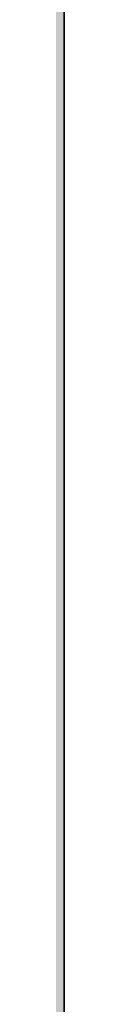
# Model space of a CAD drawing. Units: inches. Extents: x 2083 to 3317, y 1141 to 2115.
# Tile 236 of 256: x 3126.96 to 3126.96, y 1267.234 to 1271.372. Entities that reach past the tile are written whole.
import ezdxf

# ---------------------------------------------------------------- set-up
doc = ezdxf.new("R2010")
doc.units = ezdxf.units.IN
doc.layers.add('A-ANNO-DIMS', color=2, linetype='Continuous', lineweight=18)
doc.layers.add('A-WALL', color=7, linetype='Continuous', lineweight=35)
doc.layers.add('A-WALL-PATT', color=251, linetype='Continuous', lineweight=13, true_color=0x636466)
doc.styles.get("Standard").update_dxf_attribs({"font": 'arial.ttf'})
doc.dimstyles.new('ISO-25', dxfattribs={"dimtxt": 12, "dimasz": 12, "dimexe": 1.25, "dimexo": 0.625, "dimtad": 1, "dimlunit": 3, "dimtxsty": 'Standard', "dimcen": 2.5, "dimadec": 0, "dimazin": 0, "dimtfac": 1, "dimtmove": 0, "dimatfit": 3, "dimfxl": 1, "dimarcsym": 0})

# ---------------------------------------------------------------- blocks, each defined once
blk = doc.blocks.new('*D9')
at = {"layer": 'A-ANNO-DIMS', "color": 0, "lineweight": -2, "transparency": 16777216}
for p, q in [((3127.5848, 1486.7614), (3190.4031, 1486.7614)), ((3189.1531, 1474.7614), (3189.1531, 1275.2614)), ((3127.5848, 1263.2614), (3190.4031, 1263.2614))]:
    blk.add_line(p, q, dxfattribs=at)
at = {"layer": 'A-ANNO-DIMS', "color": 0, "transparency": 16777216}
for points in [[(3187.1531, 1474.7614), (3191.1531, 1474.7614), (3189.1531, 1486.7614)], [(3187.1531, 1275.2614), (3191.1531, 1275.2614), (3189.1531, 1263.2614)]]:
    blk.add_solid(points, dxfattribs=at)
at = {"layer": 'Defpoints', "color": 0, "transparency": 16777216}
for p in [(3126.9598, 1486.7614), (3126.9598, 1263.2614), (3189.1531, 1263.2614)]:
    blk.add_point(p, dxfattribs=at)
at = {"layer": 'A-ANNO-DIMS', "color": 0, "transparency": 16777216, "insert": (3182.4012, 1375.0114), "char_height": 12, "attachment_point": 5, "rotation": 90}
blk.add_mtext('18\'-7.5"', dxfattribs=at)
blk = doc.blocks.new('*D26')
at = {"layer": 'A-ANNO-DIMS', "color": 0, "lineweight": -2, "transparency": 16777216}
for p, q in [((3088.9858, 1274.9151), (3088.9858, 1270.952)), ((3111.24, 1274.9151), (3111.24, 1270.952)), ((3076.9858, 1272.202), (2840.2624, 1272.202)), ((3111.24, 1272.202), (3088.9858, 1272.202)), ((3123.24, 1272.202), (3135.24, 1272.202))]:
    blk.add_line(p, q, dxfattribs=at)
at = {"layer": 'A-ANNO-DIMS', "color": 0, "transparency": 16777216}
for points in [[(3076.9858, 1274.202), (3076.9858, 1270.202), (3088.9858, 1272.202)], [(3123.24, 1274.202), (3123.24, 1270.202), (3111.24, 1272.202)]]:
    blk.add_solid(points, dxfattribs=at)
at = {"layer": 'Defpoints', "color": 0, "transparency": 16777216}
for p in [(3088.9858, 1275.5401), (3111.24, 1275.5401), (3088.9858, 1272.202)]:
    blk.add_point(p, dxfattribs=at)
at = {"layer": 'A-ANNO-DIMS', "color": 0, "transparency": 16777216, "insert": (2952.6241, 1279.0316), "char_height": 12, "attachment_point": 5}
blk.add_mtext('NIGHTSTAND 1\'-10 1/2" TYP.', dxfattribs=at)
blk = doc.blocks.new('*D27')
at = {"layer": 'A-ANNO-DIMS', "color": 0, "lineweight": -2, "transparency": 16777216}
for p, q in [((3114.5782, 1309.7943), (3114.5782, 1321.7943)), ((3111.865, 1297.7943), (3115.8282, 1297.7943)), ((3114.5782, 1297.7943), (3114.5782, 1275.5401)), ((3111.865, 1275.5401), (3115.8282, 1275.5401)), ((3114.5782, 1263.5401), (3114.5782, 1140.9886))]:
    blk.add_line(p, q, dxfattribs=at)
at = {"layer": 'A-ANNO-DIMS', "color": 0, "transparency": 16777216}
for points in [[(3112.5782, 1309.7943), (3116.5782, 1309.7943), (3114.5782, 1297.7943)], [(3112.5782, 1263.5401), (3116.5782, 1263.5401), (3114.5782, 1275.5401)]]:
    blk.add_solid(points, dxfattribs=at)
at = {"layer": 'Defpoints', "color": 0, "transparency": 16777216}
for p in [(3111.24, 1297.7943), (3111.24, 1275.5401), (3114.5782, 1275.5401)]:
    blk.add_point(p, dxfattribs=at)
at = {"layer": 'A-ANNO-DIMS', "color": 0, "transparency": 16777216, "insert": (3107.7485, 1196.2643), "char_height": 12, "attachment_point": 5, "rotation": 90}
blk.add_mtext('1\'-10 1/2" TYP.', dxfattribs=at)

msp = doc.modelspace()

# ---------------------------------------------------------------- hatches: boundary and pattern name
at = {"layer": 'A-WALL-PATT'}
h = msp.add_hatch(color=256, dxfattribs=at)
h.dxf.hatch_style = 1
h.paths.add_polyline_path([(3126.9598, 2020.7614), (2748.9598, 2020.7614), (2604.9598, 2020.7614), (2226.9598, 2020.7614), (2226.9598, 1702.7614), (2466.9598, 1702.7614), (2466.9598, 1582.7614), (2418.9598, 1582.7614), (2418.9598, 1477.7614), (2226.9598, 1477.7614), (2226.9598, 1263.2614), (2544.9598, 1263.2614), (2544.9598, 1411.7614), (2604.9598, 1411.7614), (2685.9598, 1411.7614), (2685.9598, 1420.7614), (2604.9598, 1420.7614), (2604.9598, 1573.7614), (2604.9598, 1702.7614), (2604.9598, 2011.7614), (2748.9598, 2011.7614), (2748.9598, 1702.7614), (2862.9598, 1702.7614), (2862.9598, 1621.7614), (2871.9598, 1621.7614), (2871.9598, 1702.7614), (2883.9598, 1702.7614), (2883.9598, 1706.9395, -0.026459), (2883.9598, 1711.7614), (2757.9598, 1711.7614), (2757.9598, 1807.7614), (2787.9598, 1807.7614), (2787.9598, 1812.2614), (2757.9598, 1812.2614), (2757.9598, 2011.7614), (2877.9598, 2011.7614), (2877.9598, 1812.2614), (2847.9598, 1812.2614), (2847.9598, 1807.7614), (2889.8357, 1807.7614), (2889.8357, 1812.2614), (2882.4598, 1812.2614), (2882.4598, 2011.7614), (3117.9598, 2011.7614), (3117.9598, 1812.2614), (2937.8357, 1812.2614), (2937.8357, 1807.7614), (2995.7098, 1807.7614), (2995.7098, 1796.1177), (3000.2098, 1796.1177), (3000.2098, 1807.7614), (3117.9598, 1807.7614), (3117.9598, 1711.7614), (3000.2098, 1711.7614), (3000.2098, 1760.1177), (2998.5727, 1760.1177, -0.020711), (2995.7098, 1760.1177), (2995.7098, 1711.7614), (2931.9598, 1711.7614), (2931.9598, 1702.7614), (3126.9598, 1702.7614)])
h.paths.add_polyline_path([(2471.4598, 2011.7614), (2471.4598, 1810.0114), (2462.7169, 1810.0114), (2462.7169, 1805.5114), (2505.9598, 1805.5114), (2505.9598, 1810.0114), (2475.9598, 1810.0114), (2475.9598, 2011.7614), (2595.9598, 2011.7614), (2595.9598, 1810.0114), (2565.9598, 1810.0114), (2565.9598, 1805.5114), (2595.9598, 1805.5114), (2595.9598, 1711.7614), (2235.9598, 1711.7614), (2235.9598, 1805.5114), (2353.7098, 1805.5114), (2353.7098, 1796.0542), (2358.2098, 1796.0542), (2358.2098, 1805.5114), (2414.7169, 1805.5114), (2414.7169, 1810.0114), (2235.9598, 1810.0114), (2235.9598, 2011.7614)], flags=16)
h.paths.add_polyline_path([(2270.2047, 1994.61), (2270.2047, 1970.61), (2246.2047, 1970.61), (2246.2047, 1994.61)], flags=0)
edge = h.paths.add_edge_path(flags=0)
edge.add_ellipse((2332.0274, 1899.7982), major_axis=(-3.043, 3.043), ratio=0.168252, start_angle=-161.3322, end_angle=-156.3071, ccw=False)
edge.add_ellipse((2333.082, 1898.7435), major_axis=(-1.0546, 1.0546), ratio=0.453532, start_angle=-123.371, end_angle=-94.1591)
edge = h.paths.add_edge_path(flags=0)
edge.add_ellipse((2332.0274, 1968.8763), major_axis=(3.043, 3.043), ratio=0.168252, start_angle=18.6678, end_angle=23.6929)
edge.add_spline(control_points=[(2332.9256, 1970.6911), (2332.2268, 1970.3361), (2330.8937, 1969.6589), (2328.4131, 1970.9321), (2327.2039, 1967.7487), (2324.7096, 1969.9556), (2322.5328, 1967.0124), (2320.0128, 1971.2958), (2317.6803, 1968.1578), (2316.0405, 1967.102), (2315.4269, 1966.8096)], knot_values=[0, 0, 0, 0, 2.267059, 4.324559, 6.685584, 8.878641, 11.121502, 14.300359, 17.755284, 19.732645, 19.732645, 19.732645, 19.732645], degree=3, periodic=0)
edge.add_ellipse((2332.0274, 1968.8763), major_axis=(3.043, 3.043), ratio=0.168252, start_angle=18.6678, end_angle=23.6929, ccw=False)
edge.add_ellipse((2333.082, 1969.9309), major_axis=(1.0546, 1.0546), ratio=0.453532, start_angle=56.629, end_angle=85.8409, ccw=False)
edge = h.paths.add_edge_path(flags=0)
edge.add_spline(control_points=[(2296.4283, 1967.9879), (2293.6278, 1965.3363), (2287.7036, 1959.7271), (2299.7439, 1949.9957), (2294.5326, 1935.6685), (2290.5732, 1920.6035), (2293.3941, 1909.9737), (2296.1854, 1904.9665)], knot_values=[0.099185, 0.099185, 0.099185, 0.099185, 0.345301, 0.619822, 0.982653, 1.386093, 1.810555, 1.810555, 1.810555, 1.810555], degree=3, periodic=0)
edge.add_spline(control_points=[(2296.1854, 1904.9665), (2297.3836, 1902.6193), (2298.001, 1901.9493), (2298.553, 1901.4682)], knot_values=[0.006246, 0.006246, 0.006246, 0.006246, 0.055476, 0.055476, 0.055476, 0.055476], degree=3, periodic=0)
edge.add_spline(control_points=[(2298.553, 1901.4682), (2297.2586, 1900.9232), (2295.2253, 1900.2321), (2293.0602, 1900.6142), (2292.1014, 1900.7884), (2292.0896, 1900.7906)], knot_values=[0.312835, 0.312835, 0.312835, 0.312835, 0.40178, 0.474987, 0.475903, 0.475903, 0.475903, 0.475903], degree=3, periodic=0)
edge.add_arc((2292.7936, 1904.6641), 3.937, 215.4209, 259.6982, ccw=False)
edge.add_spline(control_points=[(2289.5853, 1902.3823), (2289.4767, 1902.5351), (2289.3685, 1902.688), (2289.2609, 1902.8412)], knot_values=[0.102872, 0.102872, 0.102872, 0.102872, 0.116896, 0.116896, 0.116896, 0.116896], degree=3, periodic=0)
edge.add_spline(control_points=[(2289.2609, 1902.8412), (2288.6866, 1902.5502), (2287.64, 1902.0199), (2285.8813, 1901.874), (2283.853, 1901.5044), (2281.72, 1899.7105), (2278.467, 1899.4929), (2276.1571, 1901.8832), (2272.259, 1899.8041), (2267.7776, 1901.8432), (2262.2439, 1900.184), (2257.4149, 1901.7821), (2254.3184, 1900.7261), (2253.1783, 1900.3373)], knot_values=[0, 0, 0, 0, 1.907977, 3.477176, 5.261074, 7.972851, 11.680248, 13.717921, 16.939592, 22.789562, 27.502503, 33.595215, 37.145618, 37.145618, 37.145618, 37.145618], degree=3, periodic=0)
edge.add_line((2253.1783, 1900.3373), (2250.2442, 1902.8412))
edge.add_line((2250.2442, 1902.8412), (2250.2442, 1965.8333))
edge.add_line((2250.2442, 1965.8333), (2253.1783, 1968.3371))
edge.add_spline(control_points=[(2253.1783, 1968.3371), (2254.3184, 1967.9483), (2257.4149, 1966.8924), (2262.2439, 1968.4904), (2267.7776, 1966.8313), (2271.5267, 1968.5372), (2273.8759, 1967.8283), (2274.2067, 1967.7276)], knot_values=[0, 0, 0, 0, 0.09018, 0.244935, 0.364644, 0.513233, 0.537855, 0.537855, 0.537855, 0.537855], degree=3, periodic=0)
edge.add_arc((2274.3529, 1963.7933), 3.937, 72.0511, 92.1279, ccw=False)
edge.add_arc((2281.2969, 1985.23), 18.5963, 252.05113, 288.56572)
edge.add_arc((2292.3167, 1956.0289), 12.6461, 71.02679, 113.77822, ccw=False)
edge = h.paths.add_edge_path(flags=0)
edge.add_spline(control_points=[(2274.8994, 1951.8562), (2275.0662, 1951.6166), (2275.2327, 1951.3766), (2275.398, 1951.1359)], knot_values=[1.409916, 1.409916, 1.409916, 1.409916, 1.43159, 1.43159, 1.43159, 1.43159], degree=3, periodic=0)
edge.add_spline(control_points=[(2275.398, 1951.1359), (2275.7921, 1950.5619), (2276.1792, 1949.9838), (2276.5455, 1949.3971)], knot_values=[1.358238, 1.358238, 1.358238, 1.358238, 1.409916, 1.409916, 1.409916, 1.409916], degree=3, periodic=0)
edge.add_line((2276.5455, 1949.3971), (2277.4373, 1947.8622))
edge.add_spline(control_points=[(2277.4373, 1947.8622), (2276.3038, 1945.6731), (2274.6397, 1942.4269), (2274.6316, 1938.0939), (2272.7991, 1930.8515), (2274.3564, 1943.897), (2275.9477, 1947.9234), (2276.5455, 1949.3971)], knot_values=[0.005632, 0.005632, 0.005632, 0.005632, 0.186014, 0.266002, 0.357087, 0.59639, 0.739732, 0.739732, 0.739732, 0.739732], degree=3, periodic=0)
edge.add_spline(control_points=[(2276.5455, 1949.3971), (2276.1792, 1949.9838), (2275.7921, 1950.5619), (2275.398, 1951.1359)], knot_values=[1.358238, 1.358238, 1.358238, 1.358238, 1.409916, 1.409916, 1.409916, 1.409916], degree=3, periodic=0)
edge.add_spline(control_points=[(2275.398, 1951.1359), (2274.9425, 1950.0805), (2274.2078, 1948.0253), (2273.9346, 1944.8515), (2272.4685, 1937.6275), (2273.4662, 1945.6965), (2274.7006, 1951.0595), (2274.8994, 1951.8562)], knot_values=[0.104364, 0.104364, 0.104364, 0.104364, 0.189636, 0.269624, 0.36071, 0.600013, 0.644622, 0.644622, 0.644622, 0.644622], degree=3, periodic=0)
h.paths.add_polyline_path([(2269.1675, 1963.1276, -0.357527), (2268.1706, 1960.9764, -0.092561), (2268.1706, 1939.4363, -0.357527), (2269.1675, 1937.2851, -0.357527), (2267.0163, 1938.282, -0.164785), (2254.6856, 1938.282, -0.357527), (2252.5344, 1937.2851, -0.357527), (2253.5313, 1939.4363, -0.092561), (2253.5313, 1960.9764, -0.357527), (2252.5344, 1963.1276, -0.357527), (2254.6856, 1962.1307, -0.164785), (2267.0163, 1962.1307, -0.357527)], flags=0)
h.paths.add_polyline_path([(2248.8741, 1967.8018), (2248.8741, 1957.0277), (2249.4578, 1957.0277), (2249.4578, 1911.6468), (2248.8741, 1911.6468), (2248.8741, 1900.8727), (2246.5119, 1900.8727, 0.197327), (2244.1497, 1902.4569), (2244.1497, 1966.2176, 0.197327), (2246.5119, 1967.8018)], flags=0)
h.paths.add_polyline_path([(2269.1675, 1931.3893, -0.357527), (2268.1706, 1929.2381, -0.092561), (2268.1706, 1907.6981, -0.357527), (2269.1675, 1905.5469, -0.357527), (2267.0163, 1906.5438, -0.164785), (2254.6856, 1906.5438, -0.357527), (2252.5344, 1905.5469, -0.357527), (2253.5313, 1907.6981, -0.092561), (2253.5313, 1929.2381, -0.357527), (2252.5344, 1931.3893, -0.357527), (2254.6856, 1930.3925, -0.164785), (2267.0163, 1930.3925, -0.357527)], flags=0)
edge = h.paths.add_edge_path(flags=0)
edge.add_spline(control_points=[(2276.1969, 1906.7237), (2276.1681, 1909.0289), (2276.114, 1913.3719), (2270.5984, 1924.925), (2273.9052, 1919.0128), (2275.9217, 1916.2621), (2275.4746, 1912.4021), (2277.2579, 1910.3806), (2276.696, 1908.225), (2276.6462, 1906.813), (2276.6178, 1906.0084)], knot_values=[0, 0, 0, 0, 8.61026, 16.221274, 18.843057, 23.804898, 27.440828, 29.356102, 31.203478, 33.650687, 33.650687, 33.650687, 33.650687], degree=3, periodic=0)
edge.add_spline(control_points=[(2276.6178, 1906.0084), (2276.6233, 1905.6241), (2276.4977, 1904.6287), (2275.4418, 1903.8547), (2274.9373, 1903.0804), (2274.8591, 1902.8412)], knot_values=[0.156488, 0.156488, 0.156488, 0.156488, 0.184398, 0.231376, 0.250598, 0.250598, 0.250598, 0.250598], degree=3, periodic=0)
edge.add_line((2274.8591, 1902.8412), (2276.506, 1902.8412))
edge.add_spline(control_points=[(2276.506, 1902.8412), (2276.7883, 1903.0849), (2277.6651, 1904.1252), (2278.2495, 1904.3407), (2277.6539, 1908.5274), (2278.1557, 1906.2278), (2278.1005, 1905.2859), (2278.8467, 1904.069), (2277.8568, 1903.4149), (2277.8742, 1902.991), (2277.9036, 1902.8412)], knot_values=[0.059574, 0.059574, 0.059574, 0.059574, 0.080753, 0.103741, 0.16972, 0.176036, 0.207137, 0.240474, 0.262341, 0.27366, 0.27366, 0.27366, 0.27366], degree=3, periodic=0)
edge.add_line((2277.9036, 1902.8412), (2280.0298, 1902.8412))
edge.add_spline(control_points=[(2280.0298, 1902.8412), (2279.8882, 1903.0884), (2279.4993, 1903.9816), (2280.1523, 1905.9393), (2278.1036, 1909.6578), (2279.7624, 1907.1853), (2280.3279, 1904.8749), (2280.4851, 1903.4896), (2281.4633, 1903.2494), (2281.7583, 1902.9365), (2281.834, 1902.8412)], knot_values=[0.013856, 0.013856, 0.013856, 0.013856, 0.034874, 0.088867, 0.107879, 0.126738, 0.158714, 0.193757, 0.217487, 0.226722, 0.226722, 0.226722, 0.226722], degree=3, periodic=0)
edge.add_spline(control_points=[(2281.834, 1902.8412), (2281.7875, 1902.8267), (2281.647, 1902.783), (2281.3955, 1902.8595), (2281.0881, 1902.9852), (2280.7207, 1903.0609), (2280.3335, 1903.0257), (2280.1248, 1902.8989), (2280.0298, 1902.8412)], knot_values=[0, 0, 0, 0, 0.14413, 0.435517, 0.749276, 1.153046, 1.548371, 1.878348, 1.878348, 1.878348, 1.878348], degree=3, periodic=0)
edge.add_line((2280.0298, 1902.8412), (2277.9036, 1902.8412))
edge.add_spline(control_points=[(2277.9036, 1902.8412), (2277.8929, 1902.7959), (2277.8654, 1902.6796), (2277.6075, 1902.6875), (2277.2741, 1902.8007), (2276.8379, 1902.6198), (2276.5838, 1902.7893), (2276.506, 1902.8412)], knot_values=[0, 0, 0, 0, 0.127189, 0.326199, 0.628009, 1.24357, 1.515331, 1.515331, 1.515331, 1.515331], degree=3, periodic=0)
edge.add_line((2276.506, 1902.8412), (2274.8591, 1902.8412))
edge.add_spline(control_points=[(2274.8591, 1902.8412), (2274.8144, 1902.8986), (2274.7251, 1903.0134), (2274.4935, 1903.119), (2274.2443, 1902.9605), (2273.9371, 1903.1849), (2273.614, 1902.9831), (2273.4083, 1902.883), (2273.3223, 1902.8412)], knot_values=[0, 0, 0, 0, 0.21843, 0.436957, 0.687977, 0.990379, 1.398396, 1.69185, 1.69185, 1.69185, 1.69185], degree=3, periodic=0)
edge.add_spline(control_points=[(2273.3223, 1902.8412), (2273.6167, 1903.4457), (2274.274, 1904.5383), (2276.0272, 1904.5737), (2276.207, 1906.5836), (2276.1969, 1906.7237)], knot_values=[0.012227, 0.012227, 0.012227, 0.012227, 0.059472, 0.106218, 0.134458, 0.134458, 0.134458, 0.134458], degree=3, periodic=0)
h.paths.add_polyline_path([(2270.7761, 1897.7898), (2270.7761, 1873.7898), (2246.7761, 1873.7898), (2246.7761, 1897.7898)], flags=0)
h.paths.add_polyline_path([(2353.7098, 1760.0051), (2353.7098, 1760.0542), (2358.2098, 1760.0542, -0.033729)], flags=0)
h.paths.add_polyline_path([(2321.8191, 1737.5292), (2341.9953, 1737.5292, -0.414214), (2343.2033, 1736.3212), (2343.2033, 1721.0206, -0.414214), (2341.9953, 1719.8127), (2321.8191, 1719.8127, -0.414214), (2320.6112, 1721.0206), (2320.6112, 1736.3212, -0.414214)], flags=0)
h.paths.add_polyline_path([(2324.235, 1736.3212), (2339.5794, 1736.3212, -0.414214), (2341.9953, 1733.9053), (2341.9953, 1725.4497, -0.414214), (2339.5794, 1723.0338), (2333.6806, 1723.0338), (2333.8453, 1722.0455, -0.870646), (2335.4254, 1721.8259, -0.767327), (2333.9227, 1721.4232), (2331.291, 1721.4232, -0.767327), (2329.7883, 1721.8259, -0.870646), (2331.3684, 1722.0455), (2331.5331, 1723.0338), (2324.235, 1723.0338, -0.414214), (2321.8191, 1725.4497), (2321.8191, 1733.9053, -0.414214)], flags=0)
h.paths.add_polyline_path([(2570.4838, 1928.6154), (2589.6838, 1928.6154), (2590.1688, 1928.6154), (2590.1688, 1904.9934), (2570.4838, 1904.9934)], flags=0)
h.paths.add_polyline_path([(2574.4473, 1927.2638, -1), (2572.8288, 1927.2638, -1)], flags=0)
h.paths.add_polyline_path([(2573.0899, 1926.9409), (2573.925, 1927.776), (2574.1477, 1927.5533), (2573.3126, 1926.7182)], flags=0)
h.paths.add_polyline_path([(2578.7791, 1919.7296, -1), (2571.5917, 1919.7296, -1)], flags=0)
h.paths.add_polyline_path([(2578.3854, 1919.7296, -1), (2571.9854, 1919.7296, -1)], flags=0)
h.paths.add_polyline_path([(2331.5958, 1729.4762, -1), (2333.618, 1729.4762, -1)], flags=0)
h.paths.add_polyline_path([(2578.0342, 1927.2638, -1), (2576.4157, 1927.2638, -1)], flags=0)
h.paths.add_polyline_path([(2576.6889, 1927.5311), (2576.9116, 1927.7538), (2577.7467, 1926.9186), (2577.524, 1926.6959)], flags=0)
h.paths.add_polyline_path([(2578.1391, 1909.8595, -1), (2572.2317, 1909.8595, -1)], flags=0)
h.paths.add_polyline_path([(2577.7454, 1909.8595, -1), (2572.6254, 1909.8595, -1)], flags=0)
h.paths.add_polyline_path([(2583.7977, 1927.2638, -1), (2582.1792, 1927.2638, -1)], flags=0)
h.paths.add_polyline_path([(2582.7186, 1927.7538), (2583.5538, 1926.9186), (2583.3311, 1926.6959), (2582.4959, 1927.5311)], flags=0)
h.paths.add_polyline_path([(2582.4959, 1927.5311), (2582.7186, 1927.7538), (2583.5538, 1926.9186), (2583.3311, 1926.6959)], flags=0)
h.paths.add_polyline_path([(2587.7391, 1920.5296, -1), (2581.8317, 1920.5296, -1)], flags=0)
h.paths.add_polyline_path([(2587.3454, 1920.5296, -1), (2582.2254, 1920.5296, -1)], flags=0)
h.paths.add_polyline_path([(2587.3846, 1927.2638, -1), (2585.7661, 1927.2638, -1)], flags=0)
h.paths.add_polyline_path([(2586.082, 1926.9802), (2586.9172, 1927.8154), (2587.1399, 1927.5927), (2586.3047, 1926.7575)], flags=0)
h.paths.add_polyline_path([(2588.3791, 1910.6595, -1), (2581.1917, 1910.6595, -1)], flags=0)
h.paths.add_polyline_path([(2587.9854, 1910.6595, -1), (2581.5854, 1910.6595, -1)], flags=0)
h.paths.add_polyline_path([(2417.1677, 1729.4779), (2437.3439, 1729.4779, -0.414214), (2438.5519, 1728.2699), (2438.5519, 1712.9693, -0.414214), (2437.3439, 1711.7614), (2417.1677, 1711.7614, -0.414214), (2415.9598, 1712.9693), (2415.9598, 1728.2699, -0.414214)], flags=0)
h.paths.add_polyline_path([(2419.5836, 1728.2699), (2434.928, 1728.2699, -0.414214), (2437.3439, 1725.8541), (2437.3439, 1717.3984, -0.414214), (2434.928, 1714.9825), (2429.0292, 1714.9825), (2429.1939, 1713.9942, -0.870646), (2430.774, 1713.7746, -0.767327), (2429.2713, 1713.372), (2426.6396, 1713.372, -0.767327), (2425.1369, 1713.7746, -0.870646), (2426.717, 1713.9942), (2426.8817, 1714.9825), (2419.5836, 1714.9825, -0.414214), (2417.1677, 1717.3984), (2417.1677, 1725.8541, -0.414214)], flags=0)
h.paths.add_polyline_path([(2419.5836, 1728.2699), (2434.928, 1728.2699, -0.414214), (2437.3439, 1725.8541), (2437.3439, 1717.3984, -0.414214), (2434.928, 1714.9825), (2429.0292, 1714.9825), (2428.3581, 1719.009), (2427.5528, 1719.009), (2426.8817, 1714.9825), (2419.5836, 1714.9825, -0.414214), (2417.1677, 1717.3984), (2417.1677, 1725.8541, -0.414214)], flags=0)
h.paths.add_polyline_path([(2426.9444, 1721.4249, -1), (2428.9666, 1721.4249, -1)], flags=0)
h.paths.add_polyline_path([(2475.9598, 1702.7614), (2595.9598, 1702.7614), (2595.9598, 1582.7614), (2475.9598, 1582.7614)], flags=16)
h.paths.add_polyline_path([(2427.9598, 1573.7614), (2595.9598, 1573.7614), (2595.9598, 1468.7614), (2595.9598, 1420.7614), (2384.4598, 1420.7614), (2384.4598, 1468.7614), (2427.9598, 1468.7614)], flags=16)
h.paths.add_polyline_path([(2379.9598, 1468.7614), (2379.9598, 1420.7614), (2235.9598, 1420.7614), (2235.9598, 1468.7614)], flags=16)
h.paths.add_polyline_path([(2317.816, 1466.6958), (2337.9922, 1466.6958, -0.414214), (2339.2002, 1465.4878), (2339.2002, 1450.1872, -0.414214), (2337.9922, 1448.9792), (2317.816, 1448.9792, -0.414214), (2316.6081, 1450.1872), (2316.6081, 1465.4878, -0.414214)], flags=0)
h.paths.add_polyline_path([(2320.2319, 1465.4878), (2335.5763, 1465.4878, -0.414214), (2337.9922, 1463.0719), (2337.9922, 1454.6163, -0.414214), (2335.5763, 1452.2004), (2329.6775, 1452.2004), (2329.8422, 1451.212, -0.870646), (2331.4223, 1450.9925, -0.767327), (2329.9196, 1450.5898), (2327.2879, 1450.5898, -0.767327), (2325.7852, 1450.9925, -0.870646), (2327.3653, 1451.212), (2327.53, 1452.2004), (2320.2319, 1452.2004, -0.414214), (2317.816, 1454.6163), (2317.816, 1463.0719, -0.414214)], flags=0)
h.paths.add_polyline_path([(2320.2319, 1465.4878), (2335.5763, 1465.4878, -0.414214), (2337.9922, 1463.0719), (2337.9922, 1454.6163, -0.414214), (2335.5763, 1452.2004), (2329.6775, 1452.2004), (2329.0064, 1456.2269), (2328.2011, 1456.2269), (2327.53, 1452.2004), (2320.2319, 1452.2004, -0.414214), (2317.816, 1454.6163), (2317.816, 1463.0719, -0.414214)], flags=0)
h.paths.add_polyline_path([(2327.5926, 1458.6428, -1), (2329.6148, 1458.6428, -1)], flags=0)
h.paths.add_polyline_path([(2244.4117, 1433.3405), (2241.9209, 1433.3405, -0.414214), (2240.0179, 1435.2435), (2240.0179, 1440.9528, -0.414211), (2241.9209, 1442.8559), (2244.4117, 1442.8559, -1.976472)], flags=0)
h.paths.add_polyline_path([(2245.3569, 1434.3975, -0.414214), (2245.3569, 1441.7988, -2.144098)], flags=0)
h.paths.add_polyline_path([(2535.9598, 1416.2614), (2535.9598, 1272.2614), (2235.9598, 1272.2614), (2235.9598, 1416.2614)], flags=16)
h.paths.add_polyline_path([(2260.1196, 1384.2928), (2260.1196, 1362.0386), (2237.8654, 1362.0386), (2237.8654, 1384.2928)], flags=0)
edge = h.paths.add_edge_path(flags=0)
edge.add_line((2318.2518, 1362.0933), (2318.1458, 1362.001))
edge.add_ellipse((2317.4451, 1360.431), major_axis=(2.8216, 2.8216), ratio=0.168252, start_angle=18.6678, end_angle=20.9481, ccw=False)
edge.add_ellipse((2318.423, 1361.409), major_axis=(0.9779, 0.9779), ratio=0.453532, start_angle=56.629, end_angle=70.2262, ccw=False)
edge = h.paths.add_edge_path(flags=0)
edge.add_line((2319.1074, 1295.5711), (2319.015, 1295.6771))
edge.add_ellipse((2317.4451, 1296.3778), major_axis=(-2.8216, 2.8216), ratio=0.168252, start_angle=-161.3322, end_angle=-159.0519, ccw=False)
edge.add_ellipse((2318.423, 1295.3999), major_axis=(-0.9779, 0.9779), ratio=0.453532, start_angle=-123.371, end_angle=-109.7738)
edge = h.paths.add_edge_path(flags=0)
edge.add_spline(control_points=[(2284.2103, 1301.1702), (2284.5807, 1300.4447), (2284.8912, 1299.892), (2285.1596, 1299.461)], knot_values=[0.039066, 0.039066, 0.039066, 0.039066, 0.055476, 0.055476, 0.055476, 0.055476], degree=3, periodic=0)
edge.add_line((2285.1596, 1299.461), (2284.2103, 1301.1702))
edge = h.paths.add_edge_path(flags=0)
edge.add_line((2280.4125, 1297.298), (2283.37, 1297.0361))
edge.add_line((2283.37, 1297.0361), (2286.4057, 1297.9263))
edge.add_spline(control_points=[(2286.4057, 1297.9263), (2285.3055, 1297.4631), (2284.3448, 1297.1292), (2283.37, 1297.0361)], knot_values=[0.394369, 0.394369, 0.394369, 0.394369, 0.475903, 0.475903, 0.475903, 0.475903], degree=3, periodic=0)
edge.add_spline(control_points=[(2283.37, 1297.0361), (2283.2814, 1297.0277), (2282.3163, 1296.9573), (2281.3125, 1297.1345), (2280.4234, 1297.296), (2280.4125, 1297.298)], knot_values=[0.312835, 0.312835, 0.312835, 0.312835, 0.320246, 0.393453, 0.394369, 0.394369, 0.394369, 0.394369], degree=3, periodic=0)
edge = h.paths.add_edge_path(flags=0)
edge.add_line((2284.4356, 1359.6073), (2280.4463, 1355.328))
edge.add_line((2280.4463, 1355.328), (2279.58, 1351.0178))
edge.add_line((2279.58, 1351.0178), (2282.413, 1346.5804))
edge.add_spline(control_points=[(2282.413, 1346.5804), (2283.1533, 1345.5892), (2284.2529, 1344.0289), (2284.801, 1342.3872), (2284.9352, 1341.8055)], knot_values=[1.240098, 1.240098, 1.240098, 1.240098, 1.332892, 1.382712, 1.382712, 1.382712, 1.382712], degree=3, periodic=0)
edge.add_spline(control_points=[(2284.9352, 1341.8055), (2285.3191, 1340.1406), (2285.233, 1338.4092), (2284.9099, 1336.6541)], knot_values=[1.097484, 1.097484, 1.097484, 1.097484, 1.240098, 1.240098, 1.240098, 1.240098], degree=3, periodic=0)
edge.add_spline(control_points=[(2284.9099, 1336.6541), (2284.5868, 1334.899), (2284.0267, 1333.1203), (2283.4626, 1331.3606)], knot_values=[0.95487, 0.95487, 0.95487, 0.95487, 1.097484, 1.097484, 1.097484, 1.097484], degree=3, periodic=0)
edge.add_line((2283.4626, 1331.3606), (2281.8904, 1326.1534))
edge.add_line((2281.8904, 1326.1534), (2280.7563, 1321.0561))
edge.add_line((2280.7563, 1321.0561), (2280.2992, 1316.002))
edge.add_line((2280.2992, 1316.002), (2280.7159, 1310.9501))
edge.add_line((2280.7159, 1310.9501), (2282.0281, 1305.9721))
edge.add_line((2282.0281, 1305.9721), (2284.2103, 1301.1702))
edge.add_spline(control_points=[(2284.2103, 1301.1702), (2283.3407, 1302.7302), (2282.6119, 1304.3365), (2282.0281, 1305.9721)], knot_values=[0.099185, 0.099185, 0.099185, 0.099185, 0.241799, 0.241799, 0.241799, 0.241799], degree=3, periodic=0)
edge.add_spline(control_points=[(2282.0281, 1305.9721), (2281.4443, 1307.6078), (2281.0055, 1309.2728), (2280.7159, 1310.9501)], knot_values=[0.241799, 0.241799, 0.241799, 0.241799, 0.384413, 0.384413, 0.384413, 0.384413], degree=3, periodic=0)
edge.add_spline(control_points=[(2280.7159, 1310.9501), (2280.4332, 1312.5876), (2280.2894, 1314.277), (2280.2989, 1315.962), (2280.2992, 1316.002)], knot_values=[0.384413, 0.384413, 0.384413, 0.384413, 0.523647, 0.527028, 0.527028, 0.527028, 0.527028], degree=3, periodic=0)
edge.add_spline(control_points=[(2280.2992, 1316.002), (2280.3123, 1317.687), (2280.4779, 1319.3679), (2280.7563, 1321.0561)], knot_values=[0.527028, 0.527028, 0.527028, 0.527028, 0.669642, 0.669642, 0.669642, 0.669642], degree=3, periodic=0)
edge.add_spline(control_points=[(2280.7563, 1321.0561), (2281.0346, 1322.7443), (2281.4259, 1324.4396), (2281.8904, 1326.1534)], knot_values=[0.669642, 0.669642, 0.669642, 0.669642, 0.812256, 0.812256, 0.812256, 0.812256], degree=3, periodic=0)
edge.add_spline(control_points=[(2281.8904, 1326.1534), (2282.2644, 1327.5333), (2282.7879, 1329.2618), (2283.3528, 1331.0178), (2283.4626, 1331.3606)], knot_values=[0.812256, 0.812256, 0.812256, 0.812256, 0.927087, 0.95487, 0.95487, 0.95487, 0.95487], degree=3, periodic=0)
edge.add_line((2283.4626, 1331.3606), (2284.9099, 1336.6541))
edge.add_line((2284.9099, 1336.6541), (2284.9352, 1341.8055))
edge.add_line((2284.9352, 1341.8055), (2282.413, 1346.5804))
edge.add_spline(control_points=[(2282.413, 1346.5804), (2281.2751, 1348.1038), (2280.0784, 1349.5703), (2279.58, 1351.0178)], knot_values=[1.382712, 1.382712, 1.382712, 1.382712, 1.525326, 1.525326, 1.525326, 1.525326], degree=3, periodic=0)
edge.add_spline(control_points=[(2279.58, 1351.0178), (2279.4433, 1351.4147), (2279.1363, 1352.8569), (2279.7352, 1354.2904), (2280.4463, 1355.328)], knot_values=[1.525326, 1.525326, 1.525326, 1.525326, 1.564439, 1.667941, 1.667941, 1.667941, 1.667941], degree=3, periodic=0)
edge.add_spline(control_points=[(2280.4463, 1355.328), (2281.4261, 1356.7578), (2282.9308, 1358.1826), (2284.4356, 1359.6073)], knot_values=[1.667941, 1.667941, 1.667941, 1.667941, 1.810555, 1.810555, 1.810555, 1.810555], degree=3, periodic=0)
edge.add_arc((2280.6231, 1348.5182), 11.7262, 71.02679, 113.77822)
edge.add_arc((2270.4049, 1375.5952), 17.2436, 252.05113, 288.56572, ccw=False)
edge.add_arc((2263.966, 1355.7178), 3.6506, 72.0511, 92.1279)
edge.add_arc((2263.966, 1355.7178), 3.6506, 92.1279, 177.9851)
edge.add_spline(control_points=[(2260.3176, 1355.8462), (2260.2604, 1354.2207), (2260.5513, 1350.1865), (2262.9993, 1346.7663), (2264.4727, 1344.649)], knot_values=[1.43159, 1.43159, 1.43159, 1.43159, 1.564144, 1.770695, 1.770695, 1.770695, 1.770695], degree=3, periodic=0)
edge.add_line((2264.4727, 1344.649), (2264.9356, 1343.9825))
edge.add_spline(control_points=[(2263.801, 1340.2481), (2263.8432, 1340.5141), (2264.0672, 1341.7565), (2264.5127, 1343.0025), (2264.935, 1343.9811)], knot_values=[0.53657, 0.53657, 0.53657, 0.53657, 0.559349, 0.644622, 0.644622, 0.644622, 0.644622], degree=3, periodic=0)
edge.add_spline(control_points=[(2264.935, 1343.9811), (2265.1178, 1343.715), (2265.2989, 1343.4479), (2265.4768, 1343.1794)], knot_values=[1.384077, 1.384077, 1.384077, 1.384077, 1.409916, 1.409916, 1.409916, 1.409916], degree=3, periodic=0)
edge.add_spline(control_points=[(2265.4768, 1343.1794), (2265.6546, 1342.9108), (2265.8293, 1342.6408), (2265.9991, 1342.3688)], knot_values=[1.358238, 1.358238, 1.358238, 1.358238, 1.384077, 1.384077, 1.384077, 1.384077], degree=3, periodic=0)
edge.add_line((2265.9991, 1342.3688), (2266.826, 1340.9455))
edge.add_spline(control_points=[(2266.826, 1340.9455), (2268.8944, 1337.0897), (2271.3982, 1325.843), (2270.5162, 1310.5686), (2275.9194, 1301.8606), (2277.7895, 1299.1994)], knot_values=[0.116896, 0.116896, 0.116896, 0.116896, 0.472987, 1.050969, 1.313793, 1.313793, 1.313793, 1.313793], degree=3, periodic=0)
edge.add_spline(control_points=[(2277.7895, 1299.1994), (2277.8394, 1299.1285), (2277.8894, 1299.0575), (2277.9396, 1298.9866)], knot_values=[0.109884, 0.109884, 0.109884, 0.109884, 0.116896, 0.116896, 0.116896, 0.116896], degree=3, periodic=0)
edge.add_line((2277.9396, 1298.9866), (2277.7888, 1299.1991))
edge.add_spline(control_points=[(2277.7888, 1299.1991), (2277.2566, 1298.9294), (2276.2864, 1298.4379), (2275.0394, 1298.3344), (2274.3833, 1298.2389), (2274.2153, 1298.2093)], knot_values=[33.12187, 33.12187, 33.12187, 33.12187, 35.029056, 36.598255, 37.144827, 37.144827, 37.144827, 37.144827], degree=3, periodic=0)
edge.add_line((2274.2153, 1298.2093), (2273.0731, 1297.893))
edge.add_spline(control_points=[(2273.0731, 1297.893), (2272.3229, 1297.5798), (2271.0392, 1296.5105), (2269.2484, 1296.2261), (2268.4231, 1296.3747)], knot_values=[26.532584, 26.532584, 26.532584, 26.532584, 29.198919, 31.839101, 31.839101, 31.839101, 31.839101], degree=3, periodic=0)
edge.add_line((2268.4231, 1296.3747), (2263.8785, 1297.4575))
edge.add_spline(control_points=[(2263.8785, 1297.4575), (2263.5561, 1297.3594), (2261.8603, 1296.8387), (2260.2388, 1297.2824), (2258.9335, 1297.5165)], knot_values=[15.919551, 15.919551, 15.919551, 15.919551, 16.939592, 21.226067, 21.226067, 21.226067, 21.226067], degree=3, periodic=0)
edge.add_line((2258.9335, 1297.5165), (2254.0552, 1297.329))
edge.add_spline(control_points=[(2254.0552, 1297.329), (2253.7555, 1297.2958), (2252.1137, 1297.1652), (2250.4619, 1297.5442), (2249.1297, 1297.6679)], knot_values=[5.306517, 5.306517, 5.306517, 5.306517, 6.276435, 10.613034, 10.613034, 10.613034, 10.613034], degree=3, periodic=0)
edge.add_line((2249.1297, 1297.6679), (2244.3316, 1296.8778))
edge.add_line((2244.3316, 1296.8778), (2241.611, 1299.1994))
edge.add_line((2241.611, 1299.1994), (2241.611, 1357.6094))
edge.add_line((2241.611, 1357.6094), (2244.3316, 1359.9311))
edge.add_line((2244.3316, 1359.9311), (2252.7288, 1359.5427))
edge.add_spline(control_points=[(2252.7288, 1359.5427), (2252.8709, 1359.5464), (2253.3057, 1359.5482), (2253.7398, 1359.5143), (2254.0317, 1359.4824)], knot_values=[0.233291, 0.233291, 0.233291, 0.233291, 0.244935, 0.268927, 0.268927, 0.268927, 0.268927], degree=3, periodic=0)
edge.add_line((2254.0317, 1359.4824), (2259.5872, 1359.4164))
edge.add_spline(control_points=[(2259.5872, 1359.4164), (2260.6771, 1359.6285), (2262.0732, 1359.897), (2263.5237, 1359.4593), (2263.8304, 1359.366)], knot_values=[0.422516, 0.422516, 0.422516, 0.422516, 0.513233, 0.537855, 0.537855, 0.537855, 0.537855], degree=3, periodic=0)
edge.add_arc((2263.966, 1355.7178), 3.6506, 72.0511, 92.1279, ccw=False)
edge.add_arc((2270.4049, 1375.5952), 17.2436, 252.05113, 288.56572)
edge.add_arc((2280.6231, 1348.5182), 11.7262, 71.02679, 113.77822, ccw=False)
h.paths.add_polyline_path([(2240.3405, 1359.4347), (2240.3405, 1349.4444), (2240.8818, 1349.4444), (2240.8818, 1307.3645), (2240.3405, 1307.3645), (2240.3405, 1297.3741), (2238.1502, 1297.3741, 0.197327), (2235.9598, 1298.8431), (2235.9598, 1357.9657, 0.197327), (2238.1502, 1359.4347)], flags=0)
h.paths.add_polyline_path([(2259.1578, 1355.1005, -0.357527), (2258.2334, 1353.1058, -0.092561), (2258.2334, 1333.1326, -0.357527), (2259.1578, 1331.1379, -0.357527), (2257.1631, 1332.0622, -0.164785), (2245.7293, 1332.0622, -0.357527), (2243.7346, 1331.1379, -0.357527), (2244.6589, 1333.1326, -0.092561), (2244.6589, 1353.1058, -0.357527), (2243.7346, 1355.1005, -0.357527), (2245.7293, 1354.1761, -0.164785), (2257.1631, 1354.1761, -0.357527)], flags=0)
edge = h.paths.add_edge_path(flags=0)
edge.add_line((2265.9991, 1342.3688), (2266.826, 1340.9455))
edge.add_line((2266.826, 1340.9455), (2265.3076, 1337.8141))
edge.add_line((2265.3076, 1337.8141), (2264.3582, 1334.6529))
edge.add_line((2264.3582, 1334.6529), (2264.262, 1333.7997))
edge.add_spline(control_points=[(2264.262, 1333.7997), (2264.2084, 1333.1871), (2264.1621, 1332.3655), (2264.0071, 1331.4139), (2263.969, 1331.2018)], knot_values=[0.464444, 0.464444, 0.464444, 0.464444, 0.516691, 0.531608, 0.531608, 0.531608, 0.531608], degree=3, periodic=0)
edge.add_spline(control_points=[(2263.969, 1331.2018), (2263.7745, 1330.1189), (2263.4244, 1328.7908), (2263.2574, 1328.5307), (2263.234, 1328.5146)], knot_values=[0.372682, 0.372682, 0.372682, 0.372682, 0.44885, 0.464444, 0.464444, 0.464444, 0.464444], degree=3, periodic=0)
edge.add_spline(control_points=[(2263.234, 1328.5146), (2263.0964, 1328.4202), (2263.1312, 1329.3015), (2263.275, 1330.6157)], knot_values=[0.280919, 0.280919, 0.280919, 0.280919, 0.372682, 0.372682, 0.372682, 0.372682], degree=3, periodic=0)
edge.add_spline(control_points=[(2263.275, 1330.6157), (2263.4187, 1331.93), (2263.6715, 1333.6773), (2263.9699, 1335.315)], knot_values=[0.189157, 0.189157, 0.189157, 0.189157, 0.280919, 0.280919, 0.280919, 0.280919], degree=3, periodic=0)
edge.add_spline(control_points=[(2263.9699, 1335.315), (2264.1005, 1336.0322), (2264.4188, 1337.6219), (2264.7548, 1338.8644), (2264.9474, 1339.4911)], knot_values=[0.097394, 0.097394, 0.097394, 0.097394, 0.137578, 0.189157, 0.189157, 0.189157, 0.189157], degree=3, periodic=0)
edge.add_spline(control_points=[(2264.9474, 1339.4911), (2265.29, 1340.6061), (2265.6442, 1341.494), (2265.9991, 1342.3688)], knot_values=[0.005632, 0.005632, 0.005632, 0.005632, 0.097394, 0.097394, 0.097394, 0.097394], degree=3, periodic=0)
h.paths.add_polyline_path([(2259.1578, 1325.671, -0.357527), (2258.2334, 1323.6763, -0.092561), (2258.2334, 1303.7031, -0.357527), (2259.1578, 1301.7084, -0.357527), (2257.1631, 1302.6327, -0.164785), (2245.7293, 1302.6327, -0.357527), (2243.7346, 1301.7084, -0.357527), (2244.6589, 1303.7031, -0.092561), (2244.6589, 1323.6763, -0.357527), (2243.7346, 1325.671, -0.357527), (2245.7293, 1324.7466, -0.164785), (2257.1631, 1324.7466, -0.357527)], flags=0)
edge = h.paths.add_edge_path(flags=0)
edge.add_spline(control_points=[(2261.7089, 1317.3114), (2261.6795, 1317.4176), (2261.7619, 1317.3885), (2262.4907, 1316.0899), (2262.9622, 1315.3009)], knot_values=[14.955861, 14.955861, 14.955861, 14.955861, 16.221274, 18.694826, 18.694826, 18.694826, 18.694826], degree=3, periodic=0)
edge.add_spline(control_points=[(2262.9622, 1315.3009), (2262.9904, 1315.2536), (2263.7021, 1314.0674), (2264.349, 1313.1272), (2264.7301, 1312.1642)], knot_values=[18.694826, 18.694826, 18.694826, 18.694826, 18.843057, 22.433791, 22.433791, 22.433791, 22.433791], degree=3, periodic=0)
edge.add_spline(control_points=[(2264.7301, 1312.1642), (2264.8756, 1311.7964), (2265.1769, 1310.7698), (2265.1431, 1309.5593), (2265.2477, 1308.8242)], knot_values=[22.433791, 22.433791, 22.433791, 22.433791, 23.804898, 26.172756, 26.172756, 26.172756, 26.172756], degree=3, periodic=0)
edge.add_line((2265.2477, 1308.8242), (2265.8508, 1307.1719))
edge.add_spline(control_points=[(2265.8508, 1307.1719), (2266.065, 1306.8217), (2266.3844, 1306.3322), (2266.4244, 1305.7805), (2266.4204, 1305.6112)], knot_values=[28.062562, 28.062562, 28.062562, 28.062562, 29.356102, 29.911721, 29.911721, 29.911721, 29.911721], degree=3, periodic=0)
edge.add_spline(control_points=[(2266.4204, 1305.6112), (2266.4161, 1305.4326), (2266.394, 1305.25), (2266.3648, 1305.0659)], knot_values=[29.911721, 29.911721, 29.911721, 29.911721, 30.497837, 30.497837, 30.497837, 30.497837], degree=3, periodic=0)
edge.add_line((2266.3648, 1305.0659), (2266.0662, 1302.1363))
edge.add_spline(control_points=[(2266.0662, 1302.1363), (2266.0712, 1301.78), (2265.9981, 1301.2), (2265.6633, 1300.759), (2265.5089, 1300.5859)], knot_values=[0.156488, 0.156488, 0.156488, 0.156488, 0.184398, 0.203543, 0.203543, 0.203543, 0.203543], degree=3, periodic=0)
edge.add_line((2265.5089, 1300.5859), (2264.4353, 1299.1994))
edge.add_line((2264.4353, 1299.1994), (2265.9624, 1299.1994))
edge.add_line((2265.9624, 1299.1994), (2267.336, 1301.1753))
edge.add_line((2267.336, 1301.1753), (2267.3117, 1301.9862))
edge.add_spline(control_points=[(2267.3117, 1301.9862), (2267.2611, 1302.8624), (2267.1602, 1303.7371), (2267.2715, 1303.3259)], knot_values=[0.126229, 0.126229, 0.126229, 0.126229, 0.166617, 0.166617, 0.166617, 0.166617], degree=3, periodic=0)
edge.add_spline(control_points=[(2267.2715, 1303.3259), (2267.28, 1303.2943), (2267.3098, 1303.1754), (2267.3735, 1302.8836), (2267.4061, 1302.6828), (2267.4179, 1302.601)], knot_values=[0.166617, 0.166617, 0.166617, 0.166617, 0.16972, 0.176036, 0.180765, 0.180765, 0.180765, 0.180765], degree=3, periodic=0)
edge.add_spline(control_points=[(2267.7439, 1300.9875), (2267.6876, 1301.1509), (2267.4805, 1301.6567), (2267.4838, 1302.1448), (2267.4179, 1302.601)], knot_values=[0.180765, 0.180765, 0.180765, 0.180765, 0.193767, 0.220139, 0.220139, 0.220139, 0.220139], degree=3, periodic=0)
edge.add_line((2267.4179, 1302.601), (2267.7439, 1300.9875))
edge.add_spline(control_points=[(2267.7439, 1300.9875), (2267.832, 1300.7319), (2267.932, 1300.3099), (2267.5548, 1299.9745), (2267.4294, 1299.8292)], knot_values=[0.220139, 0.220139, 0.220139, 0.220139, 0.240474, 0.25489, 0.25489, 0.25489, 0.25489], degree=3, periodic=0)
edge.add_line((2267.4294, 1299.8292), (2267.2584, 1299.1994))
edge.add_line((2267.2584, 1299.1994), (2269.23, 1299.1994))
edge.add_spline(control_points=[(2269.23, 1299.1994), (2269.0987, 1299.4287), (2268.8428, 1300.0163), (2269.0116, 1300.9159), (2268.9468, 1301.6607)], knot_values=[0.013856, 0.013856, 0.013856, 0.013856, 0.034874, 0.067073, 0.067073, 0.067073, 0.067073], degree=3, periodic=0)
edge.add_line((2268.9468, 1301.6607), (2268.4316, 1303.6031))
edge.add_spline(control_points=[(2268.4316, 1303.6031), (2268.1756, 1304.1924), (2267.5962, 1305.2513), (2268.0407, 1304.6232), (2268.2514, 1304.2824)], knot_values=[0.090155, 0.090155, 0.090155, 0.090155, 0.107879, 0.120289, 0.120289, 0.120289, 0.120289], degree=3, periodic=0)
edge.add_spline(control_points=[(2268.2514, 1304.2824), (2268.3609, 1304.1053), (2269.0578, 1302.918), (2269.3827, 1301.5904), (2269.5214, 1300.7759), (2269.5752, 1300.5558)], knot_values=[0.120289, 0.120289, 0.120289, 0.120289, 0.126738, 0.158714, 0.173506, 0.173506, 0.173506, 0.173506], degree=3, periodic=0)
edge.add_line((2269.5752, 1300.5558), (2270.6858, 1299.4213))
edge.add_spline(control_points=[(2270.6858, 1299.4213), (2270.7672, 1299.3573), (2270.8379, 1299.2814), (2270.9029, 1299.1994)], knot_values=[0.21816, 0.21816, 0.21816, 0.21816, 0.226722, 0.226722, 0.226722, 0.226722], degree=3, periodic=0)
edge.add_line((2270.9372, 1299.1929), (2270.9029, 1299.1994))
edge.add_spline(control_points=[(2270.9029, 1299.1994), (2270.8598, 1299.186), (2270.7295, 1299.1455), (2270.4963, 1299.2164), (2270.2717, 1299.3083), (2270.121, 1299.348), (2270.0633, 1299.3596)], knot_values=[0.939174, 0.939174, 0.939174, 0.939174, 1.083304, 1.374691, 1.68845, 1.878348, 1.878348, 1.878348, 1.878348], degree=3, periodic=0)
edge.add_line((2270.0633, 1299.3596), (2269.23, 1299.1994))
edge.add_line((2269.23, 1299.1994), (2267.2584, 1299.1994))
edge.add_spline(control_points=[(2267.2584, 1299.1994), (2267.2484, 1299.1574), (2267.223, 1299.0497), (2266.9838, 1299.0569), (2266.8092, 1299.1162), (2266.6769, 1299.1091), (2266.6365, 1299.1048)], knot_values=[0.757665, 0.757665, 0.757665, 0.757665, 0.884854, 1.083864, 1.385675, 1.515331, 1.515331, 1.515331, 1.515331], degree=3, periodic=0)
edge.add_spline(control_points=[(2266.6365, 1299.1048), (2266.4852, 1299.0888), (2266.2358, 1299.0171), (2266.0346, 1299.1513), (2265.9624, 1299.1994)], knot_values=[0, 0, 0, 0, 0.485905, 0.757665, 0.757665, 0.757665, 0.757665], degree=3, periodic=0)
edge.add_line((2265.9624, 1299.1994), (2264.4353, 1299.1994))
edge.add_line((2264.4353, 1299.1994), (2263.8584, 1299.3671))
edge.add_spline(control_points=[(2263.8584, 1299.3671), (2263.8189, 1299.3709), (2263.7795, 1299.3857), (2263.7401, 1299.4015)], knot_values=[0.845925, 0.845925, 0.845925, 0.845925, 0.978627, 0.978627, 0.978627, 0.978627], degree=3, periodic=0)
edge.add_line((2263.7218, 1299.3964), (2263.0103, 1299.1994))
edge.add_spline(control_points=[(2263.0103, 1299.1994), (2263.2458, 1299.6829), (2263.506, 1300.1281), (2263.8735, 1300.408)], knot_values=[0.012227, 0.012227, 0.012227, 0.012227, 0.052971, 0.052971, 0.052971, 0.052971], degree=3, periodic=0)
edge.add_spline(control_points=[(2263.8735, 1300.408), (2263.9321, 1300.4527), (2264.0842, 1300.553), (2264.2552, 1300.6242), (2264.3597, 1300.6647)], knot_values=[0.052971, 0.052971, 0.052971, 0.052971, 0.059472, 0.069086, 0.069086, 0.069086, 0.069086], degree=3, periodic=0)
edge.add_line((2264.3597, 1300.6647), (2265.1419, 1301.0778))
edge.add_line((2265.1419, 1301.0778), (2265.6758, 1302.7996))
edge.add_line((2265.6758, 1302.7996), (2265.5407, 1305.7041))
edge.add_line((2265.5407, 1305.7041), (2264.8031, 1309.3277))
edge.add_line((2264.8031, 1309.3277), (2263.0405, 1314.0918))
edge.add_spline(control_points=[(2263.0405, 1314.0918), (2262.3836, 1315.6714), (2261.796, 1316.9977), (2261.7089, 1317.3114)], knot_values=[11.216896, 11.216896, 11.216896, 11.216896, 14.955861, 14.955861, 14.955861, 14.955861], degree=3, periodic=0)
h.paths.add_polyline_path([(2871.9598, 1416.2614), (2895.91, 1416.2614), (2895.91, 1420.7614), (2871.9598, 1420.7614), (2871.9598, 1501.7614), (2862.9598, 1501.7614), (2862.9598, 1420.7614), (2805.9598, 1420.7614), (2805.9598, 1411.7614), (2862.9598, 1411.7614), (2862.9598, 1263.2614), (3126.9598, 1263.2614), (3126.9598, 1411.7614), (3126.9598, 1486.7614), (2943.9598, 1486.7614), (2943.9598, 1477.7614), (2967.8603, 1477.7614), (2967.8603, 1420.7614), (2943.91, 1420.7614), (2943.91, 1416.2614), (3117.9598, 1416.2614), (3117.9598, 1420.7614), (2972.3603, 1420.7614), (2972.3603, 1477.7614), (3117.9598, 1477.7614), (3117.9598, 1420.7614), (3117.9598, 1272.2614), (2871.9598, 1272.2614)], flags=0)
h.paths.add_polyline_path([(2457.1256, 1485.9425), (2527.6027, 1485.9425), (2527.6027, 1537.6357), (2457.1256, 1537.6357)], flags=8)
h.paths.add_polyline_path([(2481.0051, 1609.9818), (2590.7658, 1609.9818), (2590.7658, 1682.0034), (2481.0051, 1682.0034)], flags=8)
h.paths.add_polyline_path([(2483.085, 1729.1268), (2553.562, 1729.1268), (2553.562, 1780.82), (2483.085, 1780.82)], flags=8)
h = msp.add_hatch(color=256, dxfattribs=at)
h.dxf.hatch_style = 1
h.paths.add_polyline_path([(3126.9598, 1486.7614), (2943.9598, 1486.7614), (2943.9598, 1477.7614), (2967.8603, 1477.7614), (2967.8603, 1420.7614), (2943.91, 1420.7614), (2943.91, 1416.2614), (3117.9598, 1416.2614), (3117.9598, 1420.7614), (2972.3603, 1420.7614), (2972.3603, 1477.7614), (3117.9598, 1477.7614), (3117.9598, 1420.7614), (3117.9598, 1272.2614), (2871.9598, 1272.2614), (2871.9598, 1416.2614), (2895.91, 1416.2614), (2895.91, 1420.7614), (2871.9598, 1420.7614), (2871.9598, 1501.7614), (2862.9598, 1501.7614), (2862.9598, 1420.7614), (2805.9598, 1420.7614), (2805.9598, 1411.7614), (2862.9598, 1411.7614), (2862.9598, 1263.2614), (3126.9598, 1263.2614), (3126.9598, 1411.7614)])

# ---------------------------------------------------------------- linework, layer by layer
at = {"layer": 'A-WALL'}
msp.add_line((3126.9598, 1411.7614), (3126.9598, 1263.2614), dxfattribs=at)

# ---------------------------------------------------------------- dimensions: what is measured, and where the dimension line sits
at = {"layer": 'A-ANNO-DIMS'}
dim = msp.add_linear_dim(base=(3189.1531, 1263.2614), p1=(3126.9598, 1486.7614), p2=(3126.9598, 1263.2614), angle=90, dimstyle='ISO-25', override={"dimclrd": 0, "dimclre": 0, "dimclrt": 0}, dxfattribs=at)
dim.commit()
dim.dimension.update_dxf_attribs({"geometry": '*D9', "text_midpoint": (3182.4012, 1375.0114)})
for base, p1, p2, angle, text, picture, middle in [((3114.5782, 1275.5401), (3111.24, 1297.7943), (3111.24, 1275.5401), 270, '<> TYP.', '*D27', (3107.7485, 1196.2643)), ((3088.9858, 1272.202), (3111.24, 1275.5401), (3088.9858, 1275.5401), 180, 'NIGHTSTAND <> TYP.', '*D26', (2952.6241, 1279.0316))]:
    dim = msp.add_linear_dim(base=base, p1=p1, p2=p2, angle=angle, text=text, dimstyle='ISO-25', override={"dimdec": 1, "dimlfac": 1, "dimrnd": 0, "dimzin": 1, "dimdsep": 46, "dimlunit": 4, "dimfrac": 2}, dxfattribs=at)
    dim.commit()
    dim.dimension.update_dxf_attribs({"geometry": picture, "text_midpoint": middle})

doc.saveas('drawing.dxf')
